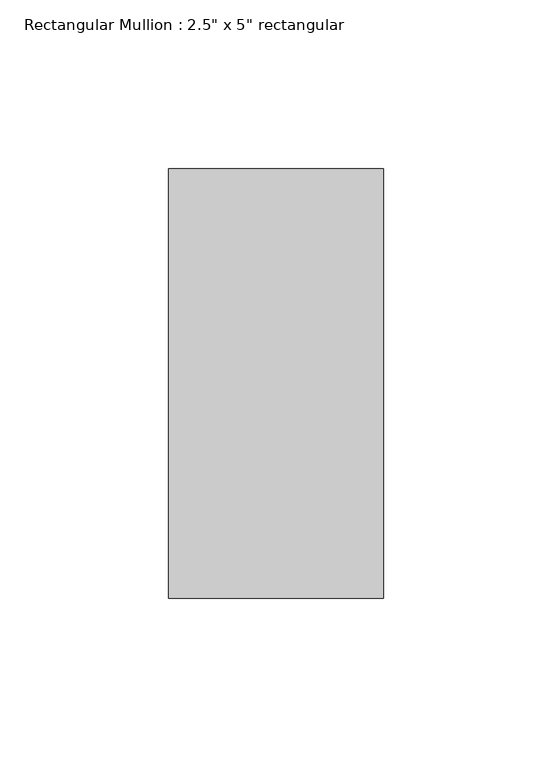
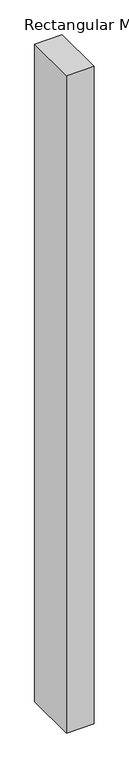
"""IFC4 building model written with IfcOpenShell, lengths in millimetres: member geometry."""

from ifc_helpers import new_model, si_unit, frame, origin, place, context, project, spatial, polyline, outline, extrude, source, transform, mapped, element, save


def member_196396ae(model_context):
    return source(origin(), model_context, "Body", "SweptSolid", [
        extrude(outline(polyline([(31.75, 63.5), (31.75, -63.5), (-31.75, -63.5), (-31.75, 63.5), (31.75, 63.5)])), frame((0.0, 0.0, -1607.0454815), z_axis=(0.0, 0.0, 1.0), x_axis=(1.0, 0.0, 0.0)), (0.0, 0.0, 1.0), 1607.0454815),
    ])


if __name__ == "__main__":
    model = new_model("IFC4")
    model_context = context("Model", 3, world=origin())
    ifc_project = project(units=[si_unit("LENGTHUNIT", "METRE", prefix="MILLI")], contexts=[model_context])
    site = spatial("IfcSite", under=ifc_project)
    building = spatial("IfcBuilding", under=site)
    placement = place(None, origin())
    member_shape = member_196396ae(model_context)
    element("IfcMember", 1, ObjectType="Rectangular Mullion : 2.5\" x 5\" rectangular", at=placement, inside=building, context=model_context, shape_type="MappedRepresentation", body=[
        mapped(member_shape, transform((0.0, 0.0, 0.0), x_axis=(1.0, 0.0, 0.0), y_axis=(0.0, 1.0, 0.0), z_axis=(0.0, 0.0, 1.0))),
    ])
    save(model, "model.ifc")

# Revit data of these elements
# Type "Rectangular Mullion : 2.5\" x 5\" rectangular"
#   built-in parameter 1007304 = 0.416667 (stored number, unit not read)
#   built-in parameter 1007301 = 0.104167 (stored number, unit not read)
#   built-in parameter 1007300 = 0.104167 (stored number, unit not read)
# Element 1 (IfcMember, "Rectangular Mullion : 2.5\" x 5\" rectangular")
#   Materials on its faces: "Aluminum"
# Materials
#   "Aluminum": class "Metal", colour RGB 247 247 247, transparency 0, Description = "Aluminum 6061", Cost = 0
